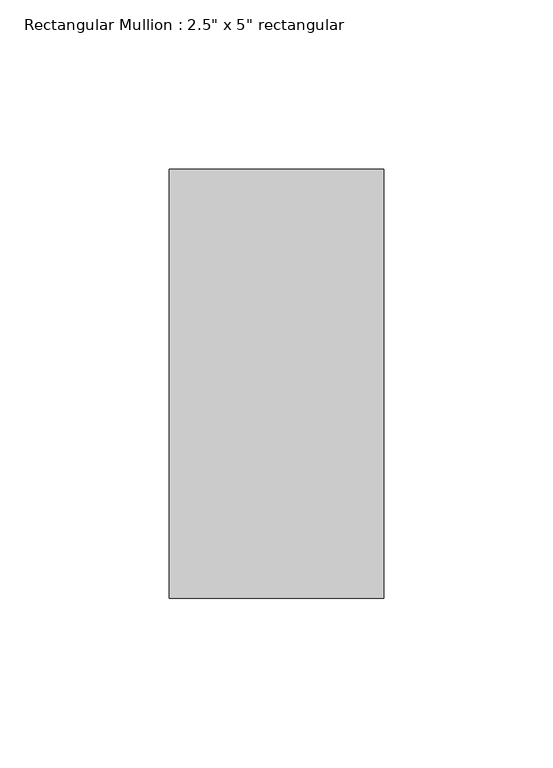
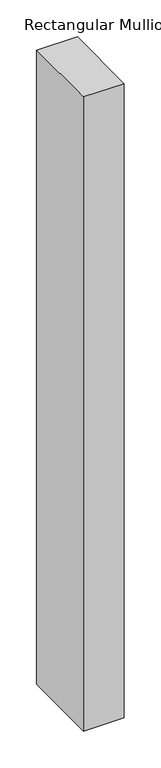
"""IFC4 building model written with IfcOpenShell, lengths in millimetres: member geometry."""

from ifc_helpers import new_model, si_unit, frame, origin, place, context, project, spatial, polyline, outline, extrude, source, transform, mapped, element, save


def member_78934672(model_context):
    return source(origin(), model_context, "Body", "SweptSolid", [
        extrude(outline(polyline([(0.0, 63.5), (0.0, -63.5), (-63.5, -63.5), (-63.5, 63.5), (0.0, 63.5)])), frame((0.0, 0.0, -1047.75), z_axis=(0.0, 0.0, 1.0), x_axis=(1.0, 0.0, 0.0)), (0.0, 0.0, 1.0), 1047.75),
    ])


if __name__ == "__main__":
    model = new_model("IFC4")
    model_context = context("Model", 3, world=origin())
    ifc_project = project(units=[si_unit("LENGTHUNIT", "METRE", prefix="MILLI")], contexts=[model_context])
    site = spatial("IfcSite", under=ifc_project)
    building = spatial("IfcBuilding", under=site)
    placement = place(None, origin())
    member_shape = member_78934672(model_context)
    element("IfcMember", 1, ObjectType="Rectangular Mullion : 2.5\" x 5\" rectangular", at=placement, inside=building, context=model_context, shape_type="MappedRepresentation", body=[
        mapped(member_shape, transform((0.0, 0.0, 0.0), x_axis=(1.0, 0.0, 0.0), y_axis=(0.0, 1.0, 0.0), z_axis=(0.0, 0.0, 1.0))),
    ])
    save(model, "model.ifc")

# Revit data of these elements
# Type "Rectangular Mullion : 2.5\" x 5\" rectangular"
#   built-in parameter 1007304 = 0.416667 (stored number, unit not read)
#   built-in parameter 1007301 = 0.104167 (stored number, unit not read)
#   built-in parameter 1007300 = 0.104167 (stored number, unit not read)
